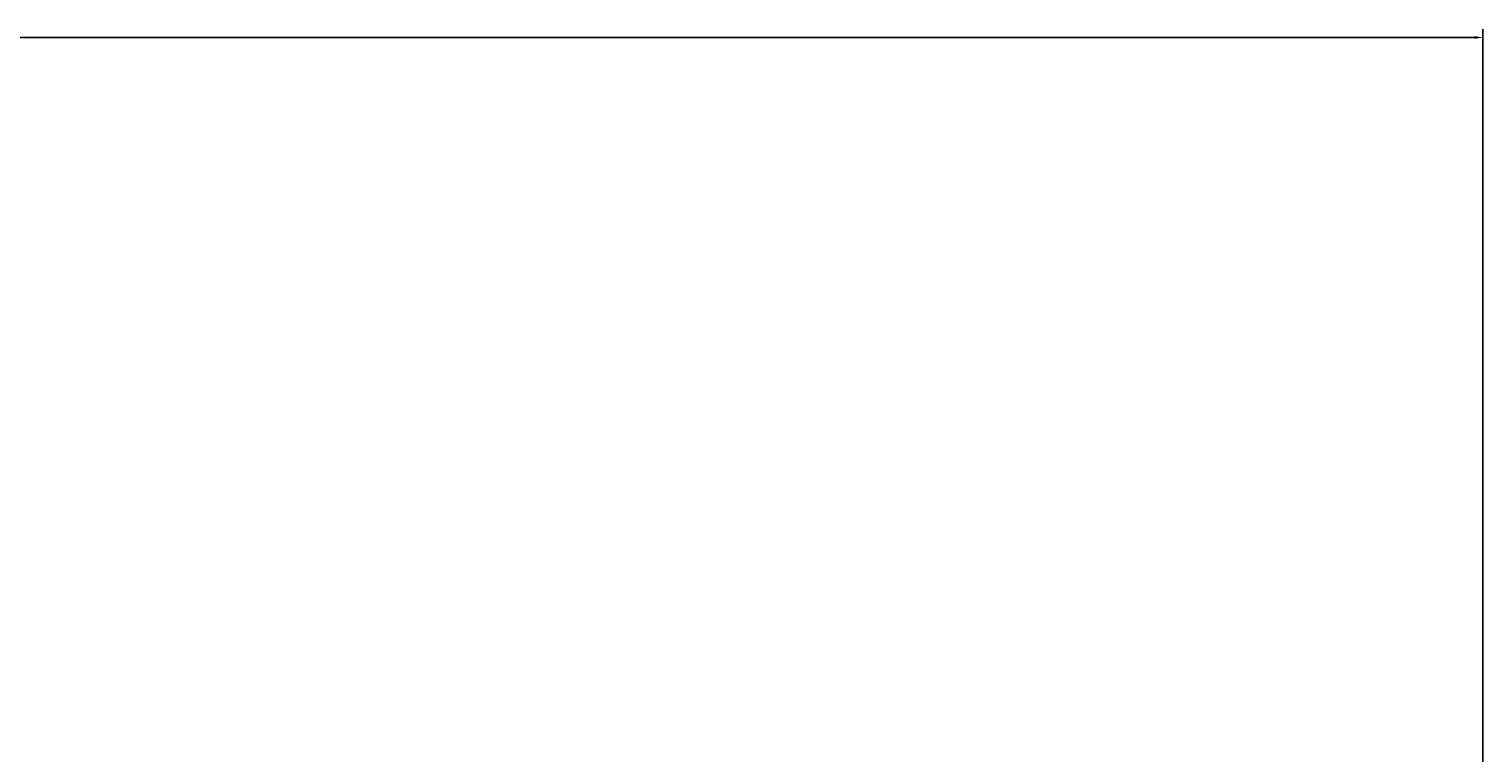
# Model space of a CAD drawing. Units: millimetres. Extents: x -9 to 135, y -119 to 27.
# Tile 12 of 12: x 95 to 126, y 11 to 27. Entities that reach past the tile are written whole.
import ezdxf

# ---------------------------------------------------------------- set-up
doc = ezdxf.new("R2010")
doc.units = ezdxf.units.MM
doc.layers.add('M-DIMS', color=2, linetype='Continuous', lineweight=18)
doc.styles.get("Standard").update_dxf_attribs({"font": 'arial.ttf'})
doc.dimstyles.get("Standard").update_dxf_attribs({"dimtxt": 0.18, "dimasz": 0.18, "dimexe": 0.18, "dimexo": 0.0625, "dimgap": 0.09, "dimtad": 0, "dimtih": 1, "dimtoh": 1, "dimdec": 4, "dimzin": 0, "dimdsep": 46, "dimtxsty": 'Standard', "dimcen": 0.09, "dimadec": 0, "dimazin": 0, "dimtfac": 1, "dimtdec": 4, "dimtofl": 0, "dimtmove": 0, "dimatfit": 3, "dimfxl": 1, "dimtolj": 1, "dimtzin": 0, "dimarcsym": 0})

# ---------------------------------------------------------------- blocks, each defined once
blk = doc.blocks.new('*D2')
at = {"layer": 'Defpoints', "color": 0, "transparency": 16777216}
for p in [(126, 26.533), (0, 17.733), (126, 1.733)]:
    blk.add_point(p, dxfattribs=at)
at = {"layer": 'M-DIMS', "color": 0, "lineweight": -2, "transparency": 16777216}
for p, q in [((0, 17.796), (0, 26.713)), ((126, 1.796), (126, 26.713)), ((0.18, 26.533), (62.72, 26.533)), ((125.82, 26.533), (63.28, 26.533))]:
    blk.add_line(p, q, dxfattribs=at)
at = {"layer": 'M-DIMS', "color": 0, "transparency": 16777216}
for points in [[(0.18, 26.563), (0.18, 26.503), (0, 26.533)], [(125.82, 26.563), (125.82, 26.503), (126, 26.533)]]:
    blk.add_solid(points, dxfattribs=at)
at = {"layer": 'M-DIMS', "color": 0, "transparency": 16777216, "insert": (63, 26.533), "char_height": 0.18, "attachment_point": 5}
blk.add_mtext('\\A1;126', dxfattribs=at)

msp = doc.modelspace()

# ---------------------------------------------------------------- dimensions: what is measured, and where the dimension line sits
at = {"layer": 'M-DIMS'}
dim = msp.add_linear_dim(base=(126, 26.533), p1=(0, 17.733), p2=(126, 1.733), dimstyle='Standard', override={"dimdec": 0, "dimlfac": 1, "dimrnd": 0, "dimzin": 0, "dimdsep": 46, "dimlunit": 2}, dxfattribs=at)
dim.commit()
dim.dimension.update_dxf_attribs({"geometry": '*D2', "text_midpoint": (63, 26.533)})

doc.saveas('drawing.dxf')
